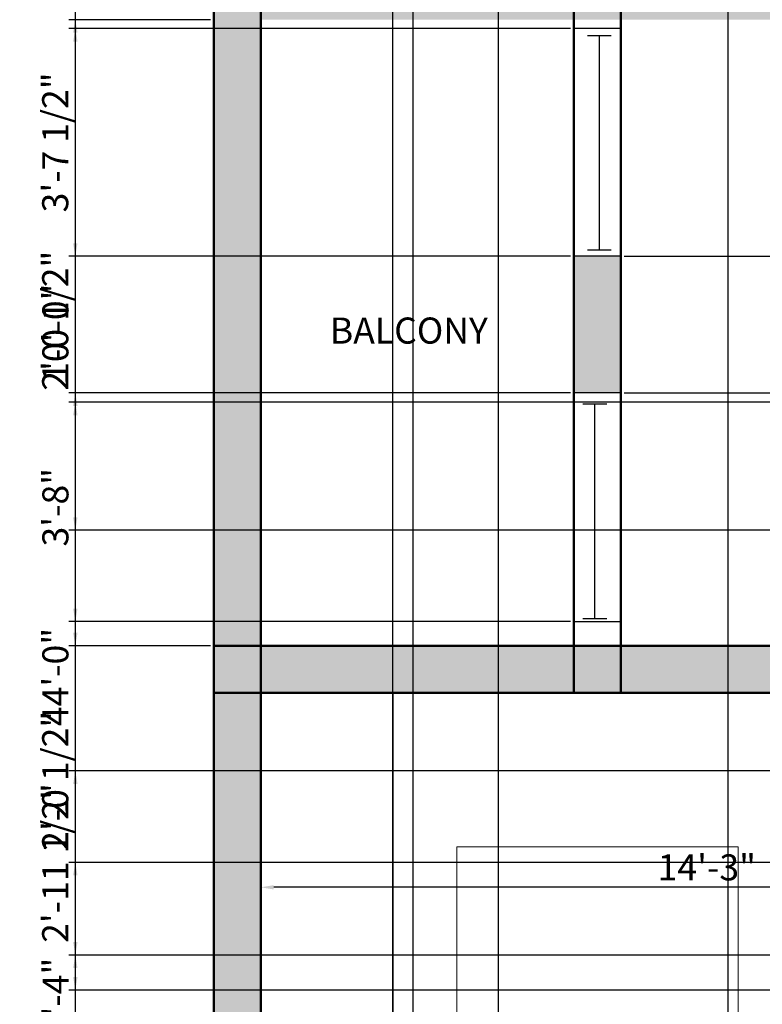
# Model space of a CAD drawing. Units: millimetres. Extents: x 2976 to 3516, y 849 to 1445.
# Tile 3 of 7: x 2976 to 3119, y 1081 to 1270. Entities that reach past the tile are written whole.
import ezdxf

# ---------------------------------------------------------------- set-up
doc = ezdxf.new("R2010")
doc.units = ezdxf.units.MM
for name, color, linetype, lineweight in [('A-AREA-IDEN', 150, 'Continuous', 25), ('A-FLOR-CASE', 130, 'Continuous', 25), ('A-WALL-PATT', 3, 'Continuous', 13), ('dimensions', 50, 'Continuous', 18), ('furniture', 130, 'Continuous', 18), ('walls', 80, 'Continuous', 50), ('windows', 10, 'Continuous', 25)]:
    doc.layers.add(name, color=color, linetype=linetype, lineweight=lineweight)
doc.styles.get("Standard").update_dxf_attribs({"font": 'arial.ttf'})
doc.dimstyles.new('ISO-25', dxfattribs={"dimtxt": 5, "dimasz": 2.5, "dimexe": 1.25, "dimexo": 0.625, "dimtad": 1, "dimdec": 0, "dimlunit": 3, "dimtxsty": 'Standard', "dimcen": 2.5, "dimadec": 0, "dimazin": 0, "dimtfac": 1, "dimtdec": 0, "dimtmove": 0, "dimatfit": 3, "dimfxl": 1, "dimarcsym": 0})

# ---------------------------------------------------------------- blocks, each defined once
blk = doc.blocks.new('*U4')
for p, q in [((0, 4), (0, 0)), ((36, 4), (36, 0)), ((0, 2), (36, 2))]:
    blk.add_line(p, q)
blk = doc.blocks.new('Bed - Queen')
for p, q in [((0, -80.00003), (0, 0)), ((0, 0), (59.99999, 0)), ((59.99999, 0), (59.99999, -80.00003)), ((7.99999, -1.2), (28.79998, -1.2)), ((7.99999, -14.4), (7.99999, -1.2)), ((28.79998, -1.2), (28.79998, -14.4)), ((31.19999, -1.2), (51.99999, -1.2)), ((31.19999, -14.4), (31.19999, -1.2)), ((51.99999, -1.2), (51.99999, -16.4)), ((0, -14.4), (44.8, -14.4)), ((59.99999, -29.6), (44.8, -14.4)), ((44.8, -14.4), (44.8, -29.6)), ((51.99999, -16.4), (46.79936, -16.4)), ((44.8, -16.8), (0, -16.8)), ((44.8, -29.6), (59.99999, -29.6)), ((59.99999, -80.00003), (0, -80.00003))]:
    blk.add_line(p, q)
blk = doc.blocks.new('*D15')
at = {"layer": 'Defpoints', "color": 0, "transparency": 16777216}
for p in [(3022.67, 1108.78), (3193.67, 1108.78), (3022.67, 1103.57)]:
    blk.add_point(p, dxfattribs=at)
at = {"layer": 'dimensions', "color": 0, "lineweight": -2, "transparency": 16777216}
for p, q in [((3022.67, 1108.16), (3022.67, 1102.32)), ((3193.67, 1108.16), (3193.67, 1102.32)), ((3191.17, 1103.57), (3025.17, 1103.57))]:
    blk.add_line(p, q, dxfattribs=at)
at = {"layer": 'dimensions', "color": 0, "transparency": 16777216}
for points in [[(3025.17, 1103.99), (3025.17, 1103.16), (3022.67, 1103.57)], [(3191.17, 1103.99), (3191.17, 1103.16), (3193.67, 1103.57)]]:
    blk.add_solid(points, dxfattribs=at)
at = {"layer": 'dimensions', "color": 0, "transparency": 16777216, "insert": (3108.17, 1106.75), "char_height": 5, "attachment_point": 5}
blk.add_mtext('14\'-3"', dxfattribs=at)
blk = doc.blocks.new('*D39')
at = {"layer": 'Defpoints', "color": 0, "transparency": 16777216}
for p in [(2987.13, 1407.88), (3013.67, 1407.88), (3013.67, 879.88)]:
    blk.add_point(p, dxfattribs=at)
at = {"layer": 'dimensions', "color": 0, "lineweight": -2, "transparency": 16777216}
for p, q in [((3013.05, 1407.88), (2985.88, 1407.88)), ((2987.13, 882.38), (2987.13, 1405.38)), ((3013.05, 879.88), (2985.88, 879.88))]:
    blk.add_line(p, q, dxfattribs=at)
at = {"layer": 'dimensions', "color": 0, "transparency": 16777216}
for points in [[(2986.71, 1405.38), (2987.55, 1405.38), (2987.13, 1407.88)], [(2986.71, 882.38), (2987.55, 882.38), (2987.13, 879.88)]]:
    blk.add_solid(points, dxfattribs=at)
at = {"layer": 'dimensions', "color": 0, "transparency": 16777216, "insert": (2983.95, 1143.88), "char_height": 5, "attachment_point": 5, "rotation": 90}
blk.add_mtext('44\'-0"', dxfattribs=at)
blk = doc.blocks.new('*D42')
at = {"layer": 'Defpoints', "color": 0, "transparency": 16777216}
for p in [(2987.13, 1269.88), (3013.67, 1269.88), (3013.67, 1149.88)]:
    blk.add_point(p, dxfattribs=at)
at = {"layer": 'dimensions', "color": 0, "lineweight": -2, "transparency": 16777216}
for p, q in [((3013.05, 1269.88), (2985.88, 1269.88)), ((2987.13, 1152.38), (2987.13, 1267.38)), ((3013.05, 1149.88), (2985.88, 1149.88))]:
    blk.add_line(p, q, dxfattribs=at)
at = {"layer": 'dimensions', "color": 0, "transparency": 16777216}
for points in [[(2986.71, 1267.38), (2987.55, 1267.38), (2987.13, 1269.88)], [(2986.71, 1152.38), (2987.55, 1152.38), (2987.13, 1149.88)]]:
    blk.add_solid(points, dxfattribs=at)
at = {"layer": 'dimensions', "color": 0, "transparency": 16777216, "insert": (2983.95, 1209.88), "char_height": 5, "attachment_point": 5, "rotation": 90}
blk.add_mtext('10\'-0"', dxfattribs=at)
blk = doc.blocks.new('*D43')
at = {"layer": 'Defpoints', "color": 0, "transparency": 16777216}
for p in [(3082.67, 1434.42), (3022.67, 1140.88), (3082.67, 1140.88)]:
    blk.add_point(p, dxfattribs=at)
at = {"layer": 'dimensions', "color": 0, "lineweight": -2, "transparency": 16777216}
for p, q in [((3022.67, 1141.51), (3022.67, 1435.67)), ((3025.17, 1434.42), (3080.17, 1434.42)), ((3082.67, 1141.51), (3082.67, 1435.67))]:
    blk.add_line(p, q, dxfattribs=at)
at = {"layer": 'dimensions', "color": 0, "transparency": 16777216}
for points in [[(3025.17, 1434.84), (3025.17, 1434), (3022.67, 1434.42)], [(3080.17, 1434.84), (3080.17, 1434), (3082.67, 1434.42)]]:
    blk.add_solid(points, dxfattribs=at)
at = {"layer": 'dimensions', "color": 0, "transparency": 16777216, "insert": (3052.67, 1437.6), "char_height": 5, "attachment_point": 5}
blk.add_mtext('5\'-0"', dxfattribs=at)
blk = doc.blocks.new('*D44')
at = {"layer": 'Defpoints', "color": 0, "transparency": 16777216}
for p in [(3242.67, 1434.42), (3091.67, 1224.53), (3242.67, 1209.88)]:
    blk.add_point(p, dxfattribs=at)
at = {"layer": 'dimensions', "color": 0, "lineweight": -2, "transparency": 16777216}
for p, q in [((3091.67, 1225.16), (3091.67, 1435.67)), ((3094.17, 1434.42), (3240.17, 1434.42)), ((3242.67, 1210.51), (3242.67, 1435.67))]:
    blk.add_line(p, q, dxfattribs=at)
at = {"layer": 'dimensions', "color": 0, "transparency": 16777216}
for points in [[(3094.17, 1434.84), (3094.17, 1434), (3091.67, 1434.42)], [(3240.17, 1434.84), (3240.17, 1434), (3242.67, 1434.42)]]:
    blk.add_solid(points, dxfattribs=at)
at = {"layer": 'dimensions', "color": 0, "transparency": 16777216, "insert": (3167.17, 1437.56), "char_height": 5, "attachment_point": 5}
blk.add_mtext('12\'-7"', dxfattribs=at)
blk = doc.blocks.new('*D53')
at = {"layer": 'Defpoints', "color": 0, "transparency": 16777216}
for p in [(2987.13, 1090.58), (3193.67, 1090.58), (3193.67, 1074.53)]:
    blk.add_point(p, dxfattribs=at)
at = {"layer": 'dimensions', "color": 0, "lineweight": -2, "transparency": 16777216}
for p, q in [((3193.05, 1090.58), (2985.88, 1090.58)), ((2987.13, 1077.03), (2987.13, 1088.08)), ((3193.05, 1074.53), (2985.88, 1074.53))]:
    blk.add_line(p, q, dxfattribs=at)
at = {"layer": 'dimensions', "color": 0, "transparency": 16777216}
for points in [[(2986.71, 1088.08), (2987.55, 1088.08), (2987.13, 1090.58)], [(2986.71, 1077.03), (2987.55, 1077.03), (2987.13, 1074.53)]]:
    blk.add_solid(points, dxfattribs=at)
at = {"layer": 'dimensions', "color": 0, "transparency": 16777216, "insert": (2984, 1082.56), "char_height": 5, "attachment_point": 5, "rotation": 90}
blk.add_mtext('1\'-4"', dxfattribs=at)
blk = doc.blocks.new('*D57')
at = {"layer": 'Defpoints', "color": 0, "transparency": 16777216}
for p in [(3112.23, 1434.42), (3068.25, 1017.88), (3112.23, 1017.88)]:
    blk.add_point(p, dxfattribs=at)
at = {"layer": 'dimensions', "color": 0, "lineweight": -2, "transparency": 16777216}
for p, q in [((3068.25, 1018.51), (3068.25, 1435.67)), ((3070.75, 1434.42), (3109.73, 1434.42)), ((3112.23, 1018.51), (3112.23, 1435.67))]:
    blk.add_line(p, q, dxfattribs=at)
at = {"layer": 'dimensions', "color": 0, "transparency": 16777216}
for points in [[(3070.75, 1434.84), (3070.75, 1434), (3068.25, 1434.42)], [(3109.73, 1434.84), (3109.73, 1434), (3112.23, 1434.42)]]:
    blk.add_solid(points, dxfattribs=at)
at = {"layer": 'dimensions', "color": 0, "transparency": 16777216, "insert": (3090.24, 1437.6), "char_height": 5, "attachment_point": 5}
blk.add_mtext('3\'-8"', dxfattribs=at)
blk = doc.blocks.new('*D63')
at = {"layer": 'Defpoints', "color": 0, "transparency": 16777216}
for p in [(2987.13, 1196.55), (3364.14, 1196.55), (3364.14, 1172.02)]:
    blk.add_point(p, dxfattribs=at)
at = {"layer": 'dimensions', "color": 0, "lineweight": -2, "transparency": 16777216}
for p, q in [((2987.13, 1196.55), (2987.13, 1225.33)), ((3363.51, 1196.55), (2985.88, 1196.55)), ((2987.13, 1174.52), (2987.13, 1194.05)), ((3363.51, 1172.02), (2985.88, 1172.02))]:
    blk.add_line(p, q, dxfattribs=at)
at = {"layer": 'dimensions', "color": 0, "transparency": 16777216}
for points in [[(2986.71, 1194.05), (2987.55, 1194.05), (2987.13, 1196.55)], [(2986.71, 1174.52), (2987.55, 1174.52), (2987.13, 1172.02)]]:
    blk.add_solid(points, dxfattribs=at)
at = {"layer": 'dimensions', "color": 0, "transparency": 16777216, "insert": (2983.92, 1212.19), "char_height": 5, "attachment_point": 5, "rotation": 90}
blk.add_mtext('2\'-0 1/2"', dxfattribs=at)
blk = doc.blocks.new('*D67')
at = {"layer": 'Defpoints', "color": 0, "transparency": 16777216}
for p in [(2987.13, 1108.35), (3300.46, 1108.35), (3300.46, 1083.88)]:
    blk.add_point(p, dxfattribs=at)
at = {"layer": 'dimensions', "color": 0, "lineweight": -2, "transparency": 16777216}
for p, q in [((2987.13, 1108.35), (2987.13, 1137.13)), ((3299.83, 1108.35), (2985.88, 1108.35)), ((2987.13, 1086.38), (2987.13, 1105.85)), ((3299.83, 1083.88), (2985.88, 1083.88))]:
    blk.add_line(p, q, dxfattribs=at)
at = {"layer": 'dimensions', "color": 0, "transparency": 16777216}
for points in [[(2986.71, 1105.85), (2987.55, 1105.85), (2987.13, 1108.35)], [(2986.71, 1086.38), (2987.55, 1086.38), (2987.13, 1083.88)]]:
    blk.add_solid(points, dxfattribs=at)
at = {"layer": 'dimensions', "color": 0, "transparency": 16777216, "insert": (2983.92, 1123.99), "char_height": 5, "attachment_point": 5, "rotation": 90}
blk.add_mtext('2\'-0 1/2"', dxfattribs=at)
blk = doc.blocks.new('*D71')
at = {"layer": 'Defpoints', "color": 0, "transparency": 16777216}
for p in [(2987.13, 1125.88), (3193.67, 1125.88), (3193.67, 1090.58)]:
    blk.add_point(p, dxfattribs=at)
at = {"layer": 'dimensions', "color": 0, "lineweight": -2, "transparency": 16777216}
for p, q in [((3193.05, 1125.88), (2985.88, 1125.88)), ((2987.13, 1093.08), (2987.13, 1123.38)), ((3193.05, 1090.58), (2985.88, 1090.58))]:
    blk.add_line(p, q, dxfattribs=at)
at = {"layer": 'dimensions', "color": 0, "transparency": 16777216}
for points in [[(2986.71, 1123.38), (2987.55, 1123.38), (2987.13, 1125.88)], [(2986.71, 1093.08), (2987.55, 1093.08), (2987.13, 1090.58)]]:
    blk.add_solid(points, dxfattribs=at)
at = {"layer": 'dimensions', "color": 0, "transparency": 16777216, "insert": (2983.92, 1108.23), "char_height": 5, "attachment_point": 5, "rotation": 90}
blk.add_mtext('2\'-11 1/2"', dxfattribs=at)
blk = doc.blocks.new('*D75')
at = {"layer": 'Defpoints', "color": 0, "transparency": 16777216}
for p in [(3022.67, 1338.88), (3051.83, 1338.88), (3051.83, 853.34)]:
    blk.add_point(p, dxfattribs=at)
at = {"layer": 'dimensions', "color": 0, "lineweight": -2, "transparency": 16777216}
for p, q in [((3022.67, 1338.26), (3022.67, 852.09)), ((3051.83, 1338.26), (3051.83, 852.09)), ((3025.17, 853.34), (3049.33, 853.34))]:
    blk.add_line(p, q, dxfattribs=at)
at = {"layer": 'dimensions', "color": 0, "transparency": 16777216}
for points in [[(3025.17, 853.76), (3025.17, 852.92), (3022.67, 853.34)], [(3049.33, 853.76), (3049.33, 852.92), (3051.83, 853.34)]]:
    blk.add_solid(points, dxfattribs=at)
at = {"layer": 'dimensions', "color": 0, "transparency": 16777216, "insert": (3037.25, 856.52), "char_height": 5, "attachment_point": 5}
blk.add_mtext('2\'-5"', dxfattribs=at)
blk = doc.blocks.new('*D77')
at = {"layer": 'Defpoints', "color": 0, "transparency": 16777216}
for p in [(3048, 1434.42), (3022.67, 1079.38), (3048, 1079.38)]:
    blk.add_point(p, dxfattribs=at)
at = {"layer": 'dimensions', "color": 0, "lineweight": -2, "transparency": 16777216}
for p, q in [((3022.67, 1080.01), (3022.67, 1435.67)), ((3025.17, 1434.42), (3045.5, 1434.42)), ((3048, 1080.01), (3048, 1435.67)), ((3048, 1434.42), (3076.78, 1434.42))]:
    blk.add_line(p, q, dxfattribs=at)
at = {"layer": 'dimensions', "color": 0, "transparency": 16777216}
for points in [[(3025.17, 1434.84), (3025.17, 1434), (3022.67, 1434.42)], [(3045.5, 1434.84), (3045.5, 1434), (3048, 1434.42)]]:
    blk.add_solid(points, dxfattribs=at)
at = {"layer": 'dimensions', "color": 0, "transparency": 16777216, "insert": (3063.64, 1437.63), "char_height": 5, "attachment_point": 5}
blk.add_mtext('2\'-1 1/2"', dxfattribs=at)
blk = doc.blocks.new('*D79')
at = {"layer": 'Defpoints', "color": 0, "transparency": 16777216}
for p in [(3068.25, 1434.42), (3048, 1017.88), (3068.25, 1017.88)]:
    blk.add_point(p, dxfattribs=at)
at = {"layer": 'dimensions', "color": 0, "lineweight": -2, "transparency": 16777216}
for p, q in [((3048, 1018.51), (3048, 1435.67)), ((3050.5, 1434.42), (3065.75, 1434.42)), ((3068.25, 1018.51), (3068.25, 1435.67))]:
    blk.add_line(p, q, dxfattribs=at)
at = {"layer": 'dimensions', "color": 0, "transparency": 16777216}
for points in [[(3050.5, 1434.84), (3050.5, 1434), (3048, 1434.42)], [(3065.75, 1434.84), (3065.75, 1434), (3068.25, 1434.42)]]:
    blk.add_solid(points, dxfattribs=at)
at = {"layer": 'dimensions', "color": 0, "transparency": 16777216, "insert": (3058.12, 1437.6), "char_height": 5, "attachment_point": 5}
blk.add_mtext('1\'-8"', dxfattribs=at)
blk = doc.blocks.new('*D81')
at = {"layer": 'Defpoints', "color": 0, "transparency": 16777216}
for p in [(2987.13, 1268.18), (3082.67, 1268.18), (3082.67, 1224.53)]:
    blk.add_point(p, dxfattribs=at)
at = {"layer": 'dimensions', "color": 0, "lineweight": -2, "transparency": 16777216}
for p, q in [((3082.05, 1268.18), (2985.88, 1268.18)), ((2987.13, 1227.03), (2987.13, 1265.68)), ((3082.05, 1224.53), (2985.88, 1224.53))]:
    blk.add_line(p, q, dxfattribs=at)
at = {"layer": 'dimensions', "color": 0, "transparency": 16777216}
for points in [[(2986.71, 1265.68), (2987.55, 1265.68), (2987.13, 1268.18)], [(2986.71, 1227.03), (2987.55, 1227.03), (2987.13, 1224.53)]]:
    blk.add_solid(points, dxfattribs=at)
at = {"layer": 'dimensions', "color": 0, "transparency": 16777216, "insert": (2983.92, 1246.36), "char_height": 5, "attachment_point": 5, "rotation": 90}
blk.add_mtext('3\'-7 1/2"', dxfattribs=at)
blk = doc.blocks.new('*D82')
at = {"layer": 'Defpoints', "color": 0, "transparency": 16777216}
for p in [(2987.13, 1198.35), (3082.67, 1198.35), (3082.67, 1154.51)]:
    blk.add_point(p, dxfattribs=at)
at = {"layer": 'dimensions', "color": 0, "lineweight": -2, "transparency": 16777216}
for p, q in [((3082.05, 1198.35), (2985.88, 1198.35)), ((2987.13, 1157.01), (2987.13, 1195.85)), ((3082.05, 1154.51), (2985.88, 1154.51))]:
    blk.add_line(p, q, dxfattribs=at)
at = {"layer": 'dimensions', "color": 0, "transparency": 16777216}
for points in [[(2986.71, 1195.85), (2987.55, 1195.85), (2987.13, 1198.35)], [(2986.71, 1157.01), (2987.55, 1157.01), (2987.13, 1154.51)]]:
    blk.add_solid(points, dxfattribs=at)
at = {"layer": 'dimensions', "color": 0, "transparency": 16777216, "insert": (2983.95, 1176.43), "char_height": 5, "attachment_point": 5, "rotation": 90}
blk.add_mtext('3\'-8"', dxfattribs=at)
blk = doc.blocks.new('*D83')
at = {"layer": 'Defpoints', "color": 0, "transparency": 16777216}
for p in [(3091.67, 1224.53), (3512.21, 1224.53), (3091.67, 1198.35)]:
    blk.add_point(p, dxfattribs=at)
at = {"layer": 'dimensions', "color": 0, "lineweight": -2, "transparency": 16777216}
for p, q in [((3092.3, 1224.53), (3513.46, 1224.53)), ((3512.21, 1200.85), (3512.21, 1222.03)), ((3092.3, 1198.35), (3513.46, 1198.35))]:
    blk.add_line(p, q, dxfattribs=at)
at = {"layer": 'dimensions', "color": 0, "transparency": 16777216}
for points in [[(3511.79, 1222.03), (3512.63, 1222.03), (3512.21, 1224.53)], [(3511.79, 1200.85), (3512.63, 1200.85), (3512.21, 1198.35)]]:
    blk.add_solid(points, dxfattribs=at)
at = {"layer": 'dimensions', "color": 0, "transparency": 16777216, "insert": (3509.08, 1211.44), "char_height": 5, "attachment_point": 5, "rotation": 90}
blk.add_mtext('2\'-2"', dxfattribs=at)

msp = doc.modelspace()

# ---------------------------------------------------------------- hatches: boundary and pattern name
at = {"layer": 'A-WALL-PATT'}
h = msp.add_hatch(color=256, dxfattribs=at)
h.dxf.hatch_style = 1
h.paths.add_polyline_path([(3022.67, 1398.88), (3013.67, 1398.88), (3013.67, 1278.88), (3022.67, 1278.88)])
h.paths.add_polyline_path([(3082.67, 1278.88), (3022.67, 1278.88), (3022.67, 1269.88), (3082.67, 1269.88)])
h.paths.add_polyline_path([(3022.67, 1278.88), (3013.67, 1278.88), (3013.67, 1269.88), (3022.67, 1269.88)])
h.paths.add_polyline_path([(3091.67, 1278.88), (3082.67, 1278.88), (3082.67, 1269.88), (3091.67, 1269.88)])
h.paths.add_polyline_path([(3121.76, 1278.88), (3091.67, 1278.88), (3091.67, 1269.88), (3121.76, 1269.88), (3121.76, 1272.56)])
h.paths.add_polyline_path([(3022.67, 1269.88), (3013.67, 1269.88), (3013.67, 1149.88), (3022.67, 1149.88)])
h.paths.add_polyline_path([(3022.67, 1140.88), (3013.67, 1140.88), (3013.67, 1017.88), (3022.67, 1017.88)])
h.paths.add_polyline_path([(3022.67, 1149.88), (3013.67, 1149.88), (3013.67, 1140.88), (3022.67, 1140.88)])
h.paths.add_polyline_path([(3082.67, 1149.88), (3022.67, 1149.88), (3022.67, 1140.88), (3082.67, 1140.88)])
h.paths.add_polyline_path([(3091.67, 1149.88), (3082.67, 1149.88), (3082.67, 1140.88), (3091.67, 1140.88)])
h.paths.add_polyline_path([(3143.42, 1147.68), (3143.42, 1149.88), (3091.67, 1149.88), (3091.67, 1140.88), (3144.23, 1140.88, -0.059251)])
h.paths.add_polyline_path([(3193.67, 1149.88), (3172.4, 1149.88), (3172.4, 1147.68), (3172.4, 1140.88), (3193.67, 1140.88)])
h.paths.add_polyline_path([(3202.67, 1149.88), (3193.67, 1149.88), (3193.67, 1140.88), (3202.67, 1140.88)])
h.paths.add_polyline_path([(3272.67, 1149.88), (3262.67, 1149.88), (3262.67, 1140.88), (3272.67, 1140.88)])
h.paths.add_polyline_path([(3272.67, 1140.88), (3262.67, 1140.88), (3262.67, 1083.88), (3272.67, 1083.88)])
h.paths.add_polyline_path([(3202.67, 1140.88), (3193.67, 1140.88), (3193.67, 1090.58), (3195.4, 1090.58, -0.118064), (3202.67, 1088.84)])
h.paths.add_polyline_path([(3202.67, 1074.53), (3195.4, 1074.53), (3193.67, 1074.53), (3193.67, 1017.88), (3202.67, 1017.88)])
h.paths.add_polyline_path([(3202.67, 1017.88), (3193.67, 1017.88), (3193.67, 1008.88), (3202.67, 1008.88)])
h.paths.add_polyline_path([(3193.67, 1017.88), (3112.23, 1017.88), (3112.23, 1008.88), (3193.67, 1008.88)])
h.paths.add_polyline_path([(3068.25, 1017.88), (3022.67, 1017.88), (3022.67, 1008.88), (3068.25, 1008.88)])
h.paths.add_polyline_path([(3022.67, 1017.88), (3013.67, 1017.88), (3013.67, 1008.88), (3022.67, 1008.88)])
h.paths.add_polyline_path([(3272.67, 1074.88), (3262.67, 1074.88), (3262.67, 1017.88), (3271.67, 1017.88), (3272.67, 1017.88)])
h.paths.add_polyline_path([(3272.67, 1083.88), (3262.67, 1083.88), (3262.67, 1074.88), (3272.67, 1074.88)])
h.paths.add_polyline_path([(3284.41, 1082.91), (3284.41, 1083.88), (3272.67, 1083.88), (3272.67, 1074.88), (3284.41, 1074.88)])
h.paths.add_polyline_path([(3383.67, 1083.88), (3300.46, 1083.88), (3300.46, 1082.91, -0.131652), (3298.31, 1074.88), (3383.67, 1074.88)])
h.paths.add_polyline_path([(3392.67, 1083.88), (3383.67, 1083.88), (3383.67, 1074.88), (3392.67, 1074.88)])
h.paths.add_polyline_path([(3392.67, 1074.88), (3383.67, 1074.88), (3383.67, 1017.88), (3392.67, 1017.88)])
h.paths.add_polyline_path([(3392.67, 1017.88), (3383.67, 1017.88), (3383.67, 1008.88), (3392.67, 1008.88)])
h.paths.add_polyline_path([(3383.67, 1017.88), (3347.17, 1017.88), (3347.17, 1008.88), (3383.67, 1008.88)])
h.paths.add_polyline_path([(3303.78, 1017.88), (3272.67, 1017.88), (3272.67, 1008.88), (3303.78, 1008.88)])
h.paths.add_polyline_path([(3272.67, 1017.88), (3271.67, 1017.88), (3262.67, 1017.88), (3262.67, 1008.88), (3272.67, 1008.88)])
h.paths.add_polyline_path([(3262.67, 1017.88), (3243.44, 1017.88), (3243.44, 1008.88), (3262.67, 1008.88)])
h.paths.add_polyline_path([(3218.58, 1017.88), (3202.67, 1017.88), (3202.67, 1008.88), (3218.58, 1008.88)])
h.paths.add_polyline_path([(3392.67, 1209.88), (3383.67, 1209.88), (3383.67, 1083.88), (3392.67, 1083.88)])
h.paths.add_polyline_path([(3392.67, 1218.88), (3383.67, 1218.88), (3383.67, 1209.88), (3392.67, 1209.88)])
h.paths.add_polyline_path([(3392.67, 1246.1), (3383.67, 1246.1), (3383.67, 1218.88), (3392.67, 1218.88)])
h.paths.add_polyline_path([(3383.67, 1218.88), (3251.67, 1218.88), (3251.67, 1209.88), (3383.67, 1209.88)])
h.paths.add_polyline_path([(3251.67, 1287.88), (3242.67, 1287.88), (3242.67, 1218.88), (3251.67, 1218.88)])
h.paths.add_polyline_path([(3251.67, 1218.88), (3242.67, 1218.88), (3242.67, 1209.88), (3251.67, 1209.88)])
h.paths.add_polyline_path([(3251.67, 1398.88), (3242.67, 1398.88), (3242.67, 1296.88), (3251.67, 1296.88)])
h.paths.add_polyline_path([(3251.67, 1296.88), (3242.67, 1296.88), (3242.67, 1287.88), (3251.67, 1287.88)])
h.paths.add_polyline_path([(3242.67, 1296.88), (3182.67, 1296.88), (3182.67, 1287.88), (3242.67, 1287.88)])
h.paths.add_polyline_path([(3182.67, 1296.88), (3173.67, 1296.88), (3173.67, 1287.88), (3182.67, 1287.88)])
h.paths.add_polyline_path([(3182.67, 1287.88), (3173.67, 1287.88), (3173.67, 1278.88), (3182.67, 1278.88)])
h.paths.add_polyline_path([(3182.67, 1278.88), (3173.67, 1278.88), (3173.67, 1269.88), (3182.67, 1269.88)])
h.paths.add_polyline_path([(3173.67, 1278.88), (3150.05, 1278.88, -0.054989), (3150.74, 1272.56), (3150.74, 1269.88), (3173.67, 1269.88)])
h.paths.add_polyline_path([(3182.67, 1398.88), (3173.67, 1398.88), (3173.67, 1296.88), (3182.67, 1296.88)])
h.paths.add_polyline_path([(3182.67, 1407.88), (3173.67, 1407.88), (3173.67, 1398.88), (3182.67, 1398.88)])
h.paths.add_polyline_path([(3173.67, 1407.88), (3104.59, 1407.88), (3104.59, 1398.88), (3173.67, 1398.88)])
h.paths.add_polyline_path([(3060.33, 1407.88), (3022.67, 1407.88), (3022.67, 1398.88), (3060.33, 1398.88)])
h.paths.add_polyline_path([(3022.67, 1407.88), (3013.67, 1407.88), (3013.67, 1398.88), (3022.67, 1398.88)])
h.paths.add_polyline_path([(3196.7, 1407.88), (3182.67, 1407.88), (3182.67, 1398.88), (3196.7, 1398.88)])
h.paths.add_polyline_path([(3242.67, 1407.88), (3223.57, 1407.88), (3223.57, 1398.88), (3242.67, 1398.88)])
h.paths.add_polyline_path([(3251.67, 1407.88), (3242.67, 1407.88), (3242.67, 1398.88), (3251.67, 1398.88)])
h.paths.add_polyline_path([(3295.02, 1407.88), (3251.67, 1407.88), (3251.67, 1398.88), (3295.02, 1398.88)])
h.paths.add_polyline_path([(3383.67, 1407.88), (3338.5, 1407.88), (3338.5, 1398.88), (3383.67, 1398.88)])
h.paths.add_polyline_path([(3392.67, 1407.88), (3383.67, 1407.88), (3383.67, 1398.88), (3392.67, 1398.88)])
h.paths.add_polyline_path([(3392.67, 1398.88), (3383.67, 1398.88), (3383.67, 1273.3, -0.079613), (3392.67, 1275.07)])
h = msp.add_hatch(color=256, dxfattribs=at)
h.dxf.hatch_style = 1
h.paths.add_polyline_path([(3091.67, 1224.53), (3082.67, 1224.53), (3082.67, 1198.35), (3091.67, 1198.35)])

# ---------------------------------------------------------------- linework, layer by layer
at = {"layer": 'A-FLOR-CASE'}
msp.add_lwpolyline([(3022.67, 1140.88), (3048, 1140.88), (3048, 1017.88), (3022.67, 1017.88)], close=True, dxfattribs=at)
at = {"layer": 'walls'}
for p, q in [((3013.67, 1407.88), (3013.67, 1008.88)), ((3022.67, 1407.88), (3022.67, 1008.88)), ((3082.67, 1278.88), (3082.67, 1140.88)), ((3091.67, 1278.88), (3091.67, 1140.88)), ((3013.67, 1149.88), (3143.42, 1149.88)), ((3013.67, 1140.88), (3144.23, 1140.88))]:
    msp.add_line(p, q, dxfattribs=at)
at = {"layer": 'windows'}
for p, q in [((3091.67, 1268.18), (3082.67, 1268.18)), ((3091.67, 1224.53), (3082.67, 1224.53)), ((3091.67, 1198.35), (3082.67, 1198.35)), ((3082.67, 1154.51), (3091.67, 1154.51))]:
    msp.add_line(p, q, dxfattribs=at)

# ---------------------------------------------------------------- block references
at = {"layer": 'furniture', "xscale": 0.8990276149147879, "yscale": 0.8990276149147879, "zscale": 0.8990276149147879, "rotation": 180}
msp.add_blockref('Bed - Queen', (3114.2, 1039.41), dxfattribs=at)
at = {"layer": 'windows', "xscale": 1.141608635997284, "yscale": 1.141608635997284, "zscale": 1.141608635997284, "rotation": 90}
for p in [(3089.85, 1225.76), (3088.98, 1155.12)]:
    msp.add_blockref('*U4', p, dxfattribs=at)

# ---------------------------------------------------------------- texts
at = {"layer": 'A-AREA-IDEN', "insert": (3035.91, 1212.79), "char_height": 5, "attachment_point": 1}
msp.add_mtext_dynamic_manual_height_columns('BALCONY', width=39.04, gutter_width=12.5, heights=[0], dxfattribs=at)

# ---------------------------------------------------------------- dimensions: what is measured, and where the dimension line sits
at = {"layer": 'dimensions'}
for base, p1, p2, override, picture, middle in [((3048, 1434.42), (3022.67, 1079.38), (3048, 1079.38), {"dimdec": 1, "dimlfac": 1, "dimrnd": 0, "dimzin": 1, "dimdsep": 46, "dimlunit": 4, "dimfrac": 2}, '*D77', (3063.64, 1437.63)), ((3082.67, 1434.42), (3022.67, 1140.88), (3082.67, 1140.88), {"dimdec": 1, "dimlfac": 1, "dimrnd": 0, "dimzin": 1, "dimdsep": 46, "dimlunit": 4, "dimfrac": 2}, '*D43', (3052.67, 1437.6)), ((3068.248, 1434.4215), (3047.9988, 1017.8815), (3068.248, 1017.8815), {"dimdec": 1, "dimlfac": 1, "dimrnd": 0, "dimzin": 1, "dimdsep": 46, "dimlunit": 4, "dimfrac": 2}, '*D79', (3058.1234, 1437.5993)), ((3112.23, 1434.42), (3068.25, 1017.88), (3112.23, 1017.88), {"dimdec": 1, "dimlfac": 1, "dimrnd": 0, "dimzin": 1, "dimdsep": 46, "dimlunit": 4, "dimfrac": 2}, '*D57', (3090.24, 1437.6)), ((3242.67, 1434.42), (3091.67, 1224.53), (3242.67, 1209.88), {"dimdec": 1, "dimlfac": 1, "dimrnd": 0, "dimzin": 1, "dimdsep": 46, "dimlunit": 4, "dimfrac": 2}, '*D44', (3167.17, 1437.56)), ((3051.83, 853.34), (3022.67, 1338.88), (3051.83, 1338.88), {"dimdec": 1, "dimlfac": 1, "dimrnd": 0, "dimzin": 1, "dimdsep": 46, "dimlunit": 4, "dimfrac": 2}, '*D75', (3037.25, 856.52)), ((3022.67, 1103.57), (3193.67, 1108.78), (3022.67, 1108.78), {"dimclrd": 0, "dimclre": 0, "dimclrt": 0}, '*D15', (3108.17, 1106.75))]:
    dim = msp.add_linear_dim(base=base, p1=p1, p2=p2, dimstyle='ISO-25', override=override, dxfattribs=at)
    dim.commit()
    dim.dimension.update_dxf_attribs({"geometry": picture, "text_midpoint": middle})
for base, p1, p2, picture, middle in [((2987.13, 1407.88), (3013.67, 879.88), (3013.67, 1407.88), '*D39', (2983.95, 1143.88)), ((2987.13, 1269.88), (3013.67, 1149.88), (3013.67, 1269.88), '*D42', (2983.95, 1209.88)), ((2987.1315, 1268.1816), (3082.6715, 1224.5323), (3082.6715, 1268.1816), '*D81', (2983.9195, 1246.3569)), ((2987.13, 1196.55), (3364.14, 1172.02), (3364.14, 1196.55), '*D63', (2983.92, 1212.19)), ((3512.21, 1224.53), (3091.67, 1198.35), (3091.67, 1224.53), '*D83', (3509.08, 1211.44)), ((2987.13, 1198.35), (3082.67, 1154.51), (3082.67, 1198.35), '*D82', (2983.95, 1176.43)), ((2987.13, 1108.35), (3300.46, 1083.88), (3300.46, 1108.35), '*D67', (2983.92, 1123.99)), ((2987.13, 1125.88), (3193.67, 1090.58), (3193.67, 1125.88), '*D71', (2983.92, 1108.23)), ((2987.1315, 1090.5844), (3193.6715, 1074.5303), (3193.6715, 1090.5844), '*D53', (2983.9963, 1082.5574))]:
    dim = msp.add_linear_dim(base=base, p1=p1, p2=p2, angle=90, dimstyle='ISO-25', override={"dimdec": 1, "dimlfac": 1, "dimrnd": 0, "dimzin": 1, "dimdsep": 46, "dimlunit": 4, "dimfrac": 2}, dxfattribs=at)
    dim.commit()
    dim.dimension.update_dxf_attribs({"geometry": picture, "text_midpoint": middle})

doc.saveas('drawing.dxf')
